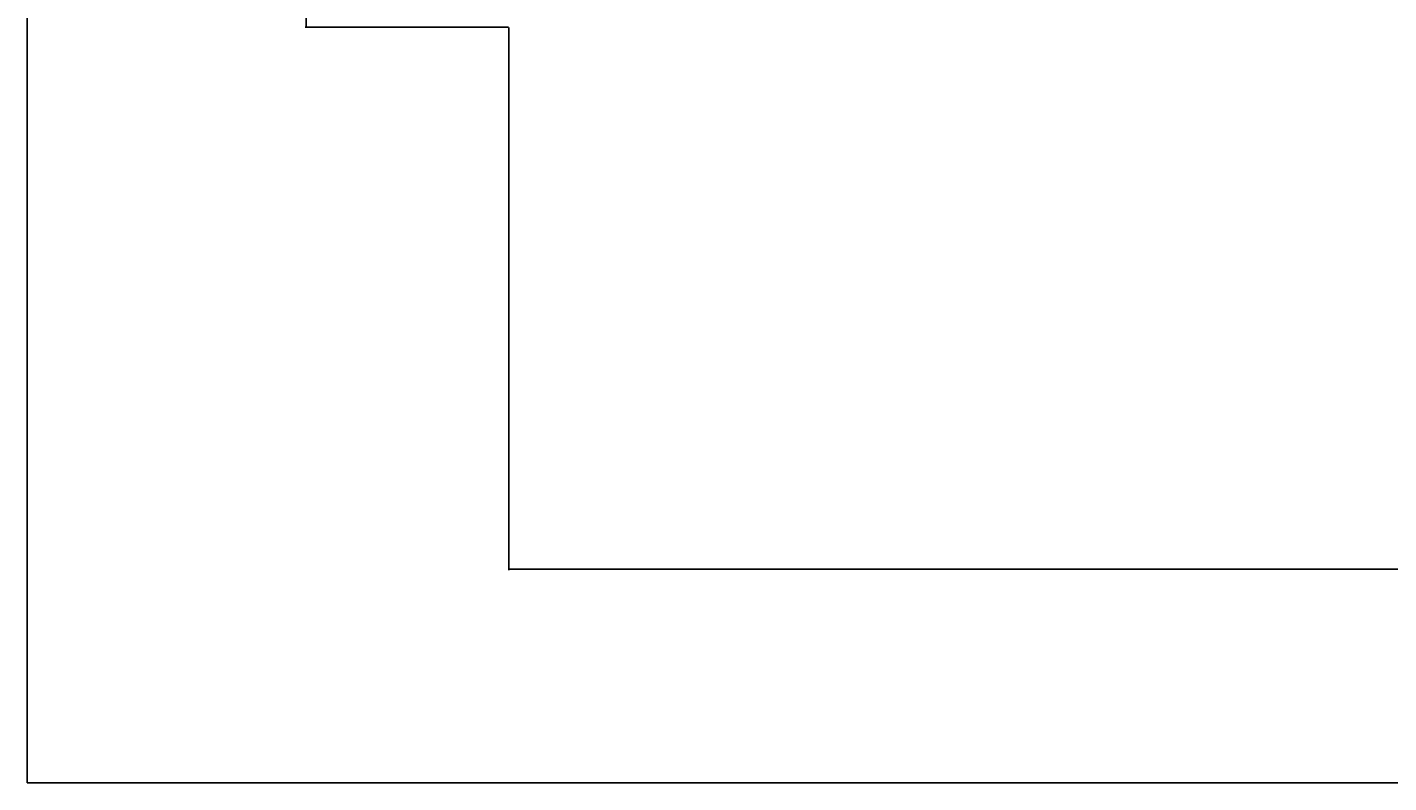
# Model space of a CAD drawing. Units: inches. Extents: x 1965 to 2673, y 1802 to 2669.
# Tile 1 of 16: x 1965 to 2198, y 1802 to 1932. Entities that reach past the tile are written whole.
import ezdxf

# ---------------------------------------------------------------- set-up
doc = ezdxf.new("R2010")
doc.units = ezdxf.units.IN
doc.layers.add('A-ANNO-DIMS', color=2, linetype='Continuous', lineweight=18)
doc.layers.add('A-ANNO-TTLB', color=7, linetype='Continuous', lineweight=25)
doc.styles.get("Standard").update_dxf_attribs({"font": 'arial.ttf'})
doc.dimstyles.get("Standard").update_dxf_attribs({"dimtxt": 0.18, "dimasz": 0.18, "dimexe": 0.18, "dimexo": 0.0625, "dimgap": 0.09, "dimtad": 0, "dimtih": 1, "dimtoh": 1, "dimdec": 4, "dimzin": 0, "dimdsep": 46, "dimtxsty": 'Standard', "dimcen": 0.09, "dimadec": 0, "dimazin": 0, "dimtfac": 1, "dimtdec": 4, "dimtofl": 0, "dimtmove": 0, "dimatfit": 3, "dimfxl": 1, "dimtolj": 1, "dimtzin": 0, "dimarcsym": 0})

# ---------------------------------------------------------------- blocks, each defined once
blk = doc.blocks.new('*D25')
at = {"layer": 'A-ANNO-DIMS', "color": 0, "lineweight": -2, "transparency": 16777216}
for p, q in [((2047.09, 1931.53), (2047.09, 1838.49)), ((2578.09, 1931.53), (2578.09, 1838.49)), ((2047.27, 1838.67), (2312.32, 1838.67)), ((2577.91, 1838.67), (2312.86, 1838.67))]:
    blk.add_line(p, q, dxfattribs=at)
at = {"layer": 'A-ANNO-DIMS', "color": 0, "transparency": 16777216}
for points in [[(2047.27, 1838.7), (2047.27, 1838.64), (2047.09, 1838.67)], [(2577.91, 1838.7), (2577.91, 1838.64), (2578.09, 1838.67)]]:
    blk.add_solid(points, dxfattribs=at)
at = {"layer": 'Defpoints', "color": 0, "transparency": 16777216}
for p in [(2047.09, 1931.59), (2578.09, 1931.59), (2578.09, 1838.67)]:
    blk.add_point(p, dxfattribs=at)
at = {"layer": 'A-ANNO-DIMS', "color": 0, "transparency": 16777216, "insert": (2312.59, 1838.67), "char_height": 0.18, "attachment_point": 5}
blk.add_mtext('\\A1;531', dxfattribs=at)
blk = doc.blocks.new('*D33')
at = {"layer": 'A-ANNO-DIMS', "color": 0, "lineweight": -2, "transparency": 16777216}
for p, q in [((2047.03, 1987.1), (2012.19, 1987.1)), ((2012.37, 1986.92), (2012.37, 1959.53)), ((2012.37, 1931.77), (2012.37, 1959.16)), ((2047.03, 1931.59), (2012.19, 1931.59))]:
    blk.add_line(p, q, dxfattribs=at)
at = {"layer": 'A-ANNO-DIMS', "color": 0, "transparency": 16777216}
for points in [[(2012.34, 1986.92), (2012.4, 1986.92), (2012.37, 1987.1)], [(2012.34, 1931.77), (2012.4, 1931.77), (2012.37, 1931.59)]]:
    blk.add_solid(points, dxfattribs=at)
at = {"layer": 'Defpoints', "color": 0, "transparency": 16777216}
for p in [(2012.37, 1987.1), (2047.09, 1987.1), (2047.09, 1931.59)]:
    blk.add_point(p, dxfattribs=at)
at = {"layer": 'A-ANNO-DIMS', "color": 0, "transparency": 16777216, "insert": (2012.37, 1959.34), "char_height": 0.18, "attachment_point": 5}
blk.add_mtext('\\A1;55.5', dxfattribs=at)

msp = doc.modelspace()

# ---------------------------------------------------------------- linework, layer by layer
at = {"layer": 'A-ANNO-TTLB'}
msp.add_lwpolyline([(1964.5703, 2669.282), (2673.2605, 2669.282), (2673.2605, 1802.0221), (1964.5703, 1802.0221)], close=True, dxfattribs=at)

# ---------------------------------------------------------------- dimensions: what is measured, and where the dimension line sits
at = {"layer": 'A-ANNO-DIMS'}
dim = msp.add_linear_dim(base=(2012.3677, 1987.096), p1=(2047.0927, 1931.5914), p2=(2047.0927, 1987.096), angle=90, dimstyle='Standard', override={"dimdec": 1, "dimlfac": 1, "dimrnd": 0, "dimzin": 0, "dimdsep": 46, "dimlunit": 2}, dxfattribs=at)
dim.commit()
dim.dimension.update_dxf_attribs({"geometry": '*D33', "text_midpoint": (2012.3677, 1959.3437)})
dim = msp.add_linear_dim(base=(2578.0927, 1838.6715), p1=(2047.0927, 1931.5914), p2=(2578.0927, 1931.5914), dimstyle='Standard', override={"dimdec": 0, "dimlfac": 1, "dimrnd": 0, "dimzin": 0, "dimdsep": 46, "dimlunit": 2}, dxfattribs=at)
dim.commit()
dim.dimension.update_dxf_attribs({"geometry": '*D25', "text_midpoint": (2312.5927, 1838.6715)})

doc.saveas('drawing.dxf')
